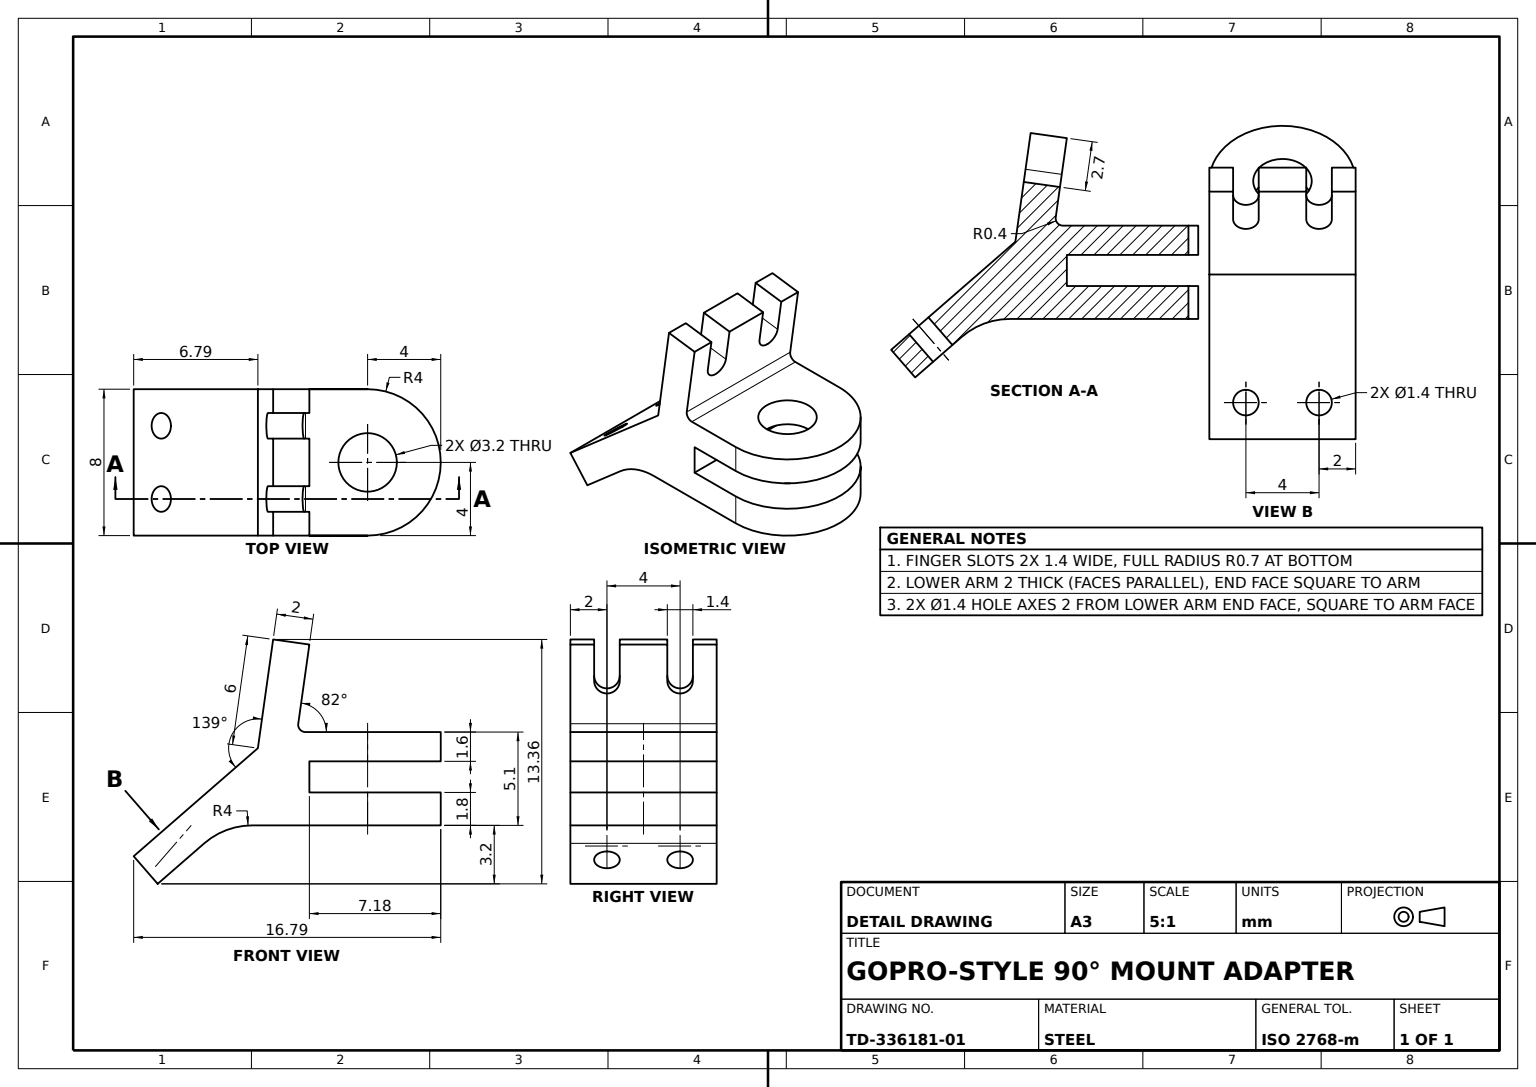
from build123d import *

# Parameters (mm, degrees)
BASE_ARM_8MM_DEPTH   = 4
FINGER_SLOTS_DEPTH   = 8
SIDE_SLOT_PROFILE_R  = 0.7
SIDE_SLOT_DEPTH      = 12.515344682
CLEVIS_LUG_8MM_DEPTH = 4
LUG_END_ROUND_R4_R   = 4
EDGE_FILLET_R0_4_R   = 0.4
LUG_FILL_BOSS_DEPTH  = 1.8
LUG_BLEND_BOSS_DEPTH = 1.6
PIN_HOLE_PROFILE_R   = 1.6
PIN_HOLE_3_2_DEPTH   = 13.647446253


with BuildPart() as part:
    # Base Arm Profile → Base Arm 8mm (new, symmetric)
    with BuildSketch(Plane.XY):
        Polygon((0, 0), (-7.356734921, -6.3951121), (-8.668852979, -4.88569294), (-1.876466757, 1.018838321), (-1.041428151, 6.960446733), (0.939107986, 6.682100531), align=None)
    extrude(amount=BASE_ARM_8MM_DEPTH, both=True)

    # Finger Slots Profile → Finger Slots (cut)
    with BuildSketch(Plane(origin=(-1.980536137, 0.278346202, 0), x_dir=(0, 0, 1), z_dir=(-0.9902680687415697, 0.13917310096006985, 0))):
        with BuildLine():
            Line((-2.7, 4.747769359), (-2.7, 6.747769359))
            Line((-2.7, 6.747769359), (-1.3, 6.747769359))
            Line((-1.3, 6.747769359), (-1.3, 4.747769359))
            ThreePointArc((-1.3, 4.747769359), (-2, 4.047769359), (-2.7, 4.747769359))
        make_face()
        with BuildLine():
            Line((1.3, 6.747769359), (1.3, 4.747769359))
            ThreePointArc((1.3, 4.747769359), (2, 4.047769359), (2.7, 4.747769359))
            Line((2.7, 4.747769359), (2.7, 6.747769359))
            Line((2.7, 6.747769359), (1.3, 6.747769359))
        make_face()
    extrude(amount=-FINGER_SLOTS_DEPTH, mode=Mode.SUBTRACT)

    # Side Slot Profile → Side Slot (cut, through all)
    with BuildSketch(Plane(origin=(-1.312118058, 1.50941916, 0), x_dir=(0.7547095802227755, 0.6560590289905035, 0), z_dir=(-0.6560590289905035, 0.7547095802227755, 0))):
        with Locations(Location((-7.747769359, -2, 0), (0, 0, 180))):
            Circle(SIDE_SLOT_PROFILE_R)
        with Locations(Location((-7.747769359, 2, 0), (0, 0, 180))):
            Circle(SIDE_SLOT_PROFILE_R)
    extrude(amount=-SIDE_SLOT_DEPTH, mode=Mode.SUBTRACT)

    # Clevis Lug Profile → Clevis Lug 8mm (add, symmetric)
    with BuildSketch(Plane.XY):
        Polygon((-3.681178903, -3.2), (4.123533243, -3.2), (4.123533243, -1.4), (0.939107986, -1.4), (0.939107986, 0.3), (4.123533243, 0.3), (4.123533243, 1.9), (0.267027586, 1.9), (0, 0), align=None)
    extrude(amount=CLEVIS_LUG_8MM_DEPTH, both=True)

    # Lug End Round R4
    lug_end_round_r4_edges = [part.edges().sort_by_distance(p)[0] for p in [
        (-3.681178903, -3.2, 0),
    ]]
    fillet(lug_end_round_r4_edges, radius=LUG_END_ROUND_R4_R)

    # Edge Fillet R0.4
    edge_fillet_r0_4_edges = [part.edges().sort_by_distance(p)[0] for p in [
        (0.267027586, 1.9, 0),
    ]]
    fillet(edge_fillet_r0_4_edges, radius=EDGE_FILLET_R0_4_R)

    # Lug Fill Boss Profile → Lug Fill Boss (add)
    with BuildSketch(Plane(origin=(0, -1.4, 0), x_dir=(1, 0, 0), z_dir=(0, 1, 0))):
        with BuildLine():
            Line((4.123533243, 4), (4.123533243, -4))
            ThreePointArc((4.123533243, -4), (8.123533243, 0), (4.123533243, 4))
        make_face()
    extrude(amount=-LUG_FILL_BOSS_DEPTH)

    # Lug Blend Boss Profile → Lug Blend Boss (add)
    with BuildSketch(Plane(origin=(0, 1.9, 0), x_dir=(1, 0, 0), z_dir=(0, 1, 0))):
        with BuildLine():
            Line((4.123533243, 4), (4.123533243, -4))
            ThreePointArc((4.123533243, -4), (8.123533243, 0), (4.123533243, 4))
        make_face()
    extrude(amount=-LUG_BLEND_BOSS_DEPTH)

    # Pin Hole Profile → Pin Hole Ø3.2 (cut, through all)
    with BuildSketch(Plane(origin=(0, 1.9, 0), x_dir=(1, 0, 0), z_dir=(0, 1, 0))):
        with Locations(Location((4.123533243, 0, 0), (0, 0, 180))):
            Circle(PIN_HOLE_PROFILE_R)
    extrude(amount=-PIN_HOLE_3_2_DEPTH, mode=Mode.SUBTRACT)


solid = part.part
